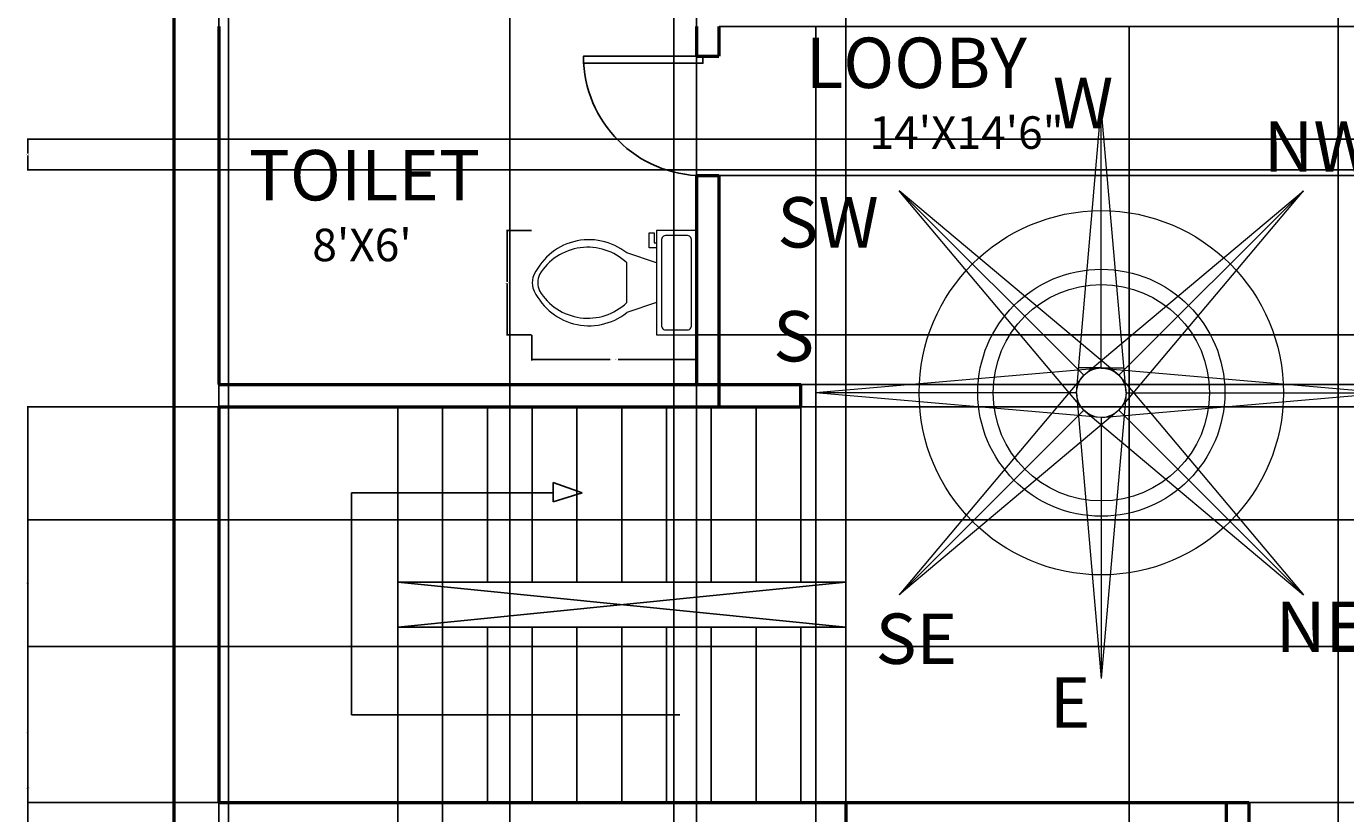
# Model space of a CAD drawing. Units: inches. Extents: x 19425 to 19848, y 45806 to 46417.
# Tile 3 of 5: x 19425 to 19690, y 45967 to 46125. Entities that reach past the tile are written whole.
import ezdxf

# ---------------------------------------------------------------- set-up
doc = ezdxf.new("R2010")
doc.units = ezdxf.units.IN
for name, color, linetype, lineweight in [('A-ANNO-DIMS', 2, 'Continuous', 18), ('A-ANNO-SYMB', 3, 'Continuous', 18), ('A-AREA-IDEN', 3, 'Continuous', 25), ('A-FLOR-FIXT', 2, 'Continuous', 20), ('door', 4, 'Continuous', 25), ('furniture', 2, 'Continuous', 18), ('staircase', 7, 'Continuous', 25), ('wall', 6, 'Continuous', 50)]:
    doc.layers.add(name, color=color, linetype=linetype, lineweight=lineweight)
doc.styles.get("Standard").update_dxf_attribs({"font": 'arial.ttf'})
doc.dimstyles.get("Standard").update_dxf_attribs({"dimtxt": 0.18, "dimasz": 0.18, "dimexe": 0.18, "dimexo": 0.0625, "dimgap": 0.09, "dimtad": 0, "dimtih": 1, "dimtoh": 1, "dimdec": 4, "dimzin": 0, "dimdsep": 46, "dimtxsty": 'Standard', "dimcen": 0.09, "dimadec": 0, "dimazin": 0, "dimtfac": 1, "dimtdec": 4, "dimtofl": 0, "dimtmove": 0, "dimatfit": 3, "dimfxl": 1, "dimtolj": 1, "dimtzin": 0, "dimarcsym": 0})

# ---------------------------------------------------------------- blocks, each defined once
blk = doc.blocks.new('*U2')
for p, q in [((0, 0), (0, -100)), ((750, 0), (750, -100))]:
    blk.add_line(p, q)
blk.add_lwpolyline([(0, 0), (0, 750), (43.75, 750), (43.75, 0)], close=True)
blk.add_arc((0, 0), 750, 0, 90)
blk = doc.blocks.new('Toilet - top')
for p, q in [((9.5, -6), (9.5, -2)), ((-10, -8.5), (-8, -8.5)), ((-10, -9.5), (-10, -8.5)), ((-7, -9.5), (-10, -9.5)), ((-8, -8.5), (-8, -8)), ((-7, -8), (-7, -9.5)), ((-4, -8), (-6, -14)), ((4, -8), (6, -14)), ((4, -14), (-4, -14))]:
    blk.add_line(p, q)
blk.add_lwpolyline([(10.5, -8), (10.5, 0), (-10.5, 0), (-10.5, -8)], close=True)
for points in [[(-9.5, -2), (-9.5, -6)], [(8.5, -1), (-8.5, -1)], [(-8.5, -7), (8.5, -7)]]:
    blk.add_lwpolyline(points)
for centre, radius, start, end in [((-8.62, -1.88), 0.884, 81.8699, 188.1301), ((8.62, -1.88), 0.884, 351.8699, 98.1301), ((-8.62, -6.12), 0.884, 171.8699, 278.1301), ((8.62, -6.12), 0.884, 261.8699, 8.1301), ((3.52, -21.58), 12.17, 141.4691, 247.9714), ((4.2, -21.82), 11.33, 136.3677, 238.9468), ((-3.52, -21.58), 12.17, 292.0284, 38.5307), ((-4.2, -21.82), 11.33, 301.053, 43.6321), ((0, -27.88), 4, 245.7318, 294.2682), ((0, -29), 4, 254.8605, 285.1395)]:
    blk.add_arc(centre, radius, start, end)
blk = doc.blocks.new('*U7')
at = {"layer": 'furniture'}
for p in [(-4.98, -28.71), (0, -23.73), (4.98, -28.71)]:
    blk.add_line(p, (0, 28.71), dxfattribs=at)
blk = doc.blocks.new('*U8')
at = {"layer": 'A-ANNO-SYMB', "transparency": 16777216}
blk.add_blockref('*U7', (19641.16, 46080.31), dxfattribs=at)
for p, rotation in [((19620.86, 46071.91), 45.00000000000001), ((19661.46, 46071.91), 315), ((19612.45, 46051.6), 90), ((19669.87, 46051.6), 270.0000000000001), ((19620.86, 46031.3), 135), ((19661.46, 46031.3), 225), ((19641.16, 46022.9), 180)]:
    blk.add_blockref('*U7', p, dxfattribs=dict(at, rotation=rotation))
blk = doc.blocks.new('*D18')
at = {"layer": 'A-ANNO-DIMS', "color": 0, "lineweight": -2, "transparency": 16777216}
for p, q in [((19526.73, 46063.16), (19526.73, 46058.08)), ((19559.78, 46063.16), (19559.78, 46058.08)), ((19526.91, 46058.26), (19542.48, 46058.26)), ((19559.6, 46058.26), (19544.03, 46058.26))]:
    blk.add_line(p, q, dxfattribs=at)
at = {"layer": 'A-ANNO-DIMS', "color": 0, "transparency": 16777216}
for points in [[(19526.91, 46058.29), (19526.91, 46058.23), (19526.73, 46058.26)], [(19559.6, 46058.29), (19559.6, 46058.23), (19559.78, 46058.26)]]:
    blk.add_solid(points, dxfattribs=at)
at = {"layer": 'Defpoints', "color": 0, "transparency": 16777216}
for p in [(19526.73, 46063.22), (19559.78, 46063.22), (19559.78, 46058.26)]:
    blk.add_point(p, dxfattribs=at)
at = {"layer": 'A-ANNO-DIMS', "color": 0, "transparency": 16777216, "insert": (19543.26, 46058.26), "char_height": 0.18, "attachment_point": 5}
blk.add_mtext('\\A1;WC 33 TYP.', dxfattribs=at)
blk = doc.blocks.new('*D19')
at = {"layer": 'A-ANNO-DIMS', "color": 0, "lineweight": -2, "transparency": 16777216}
for p, q in [((19526.67, 46084.22), (19521.6, 46084.22)), ((19521.78, 46084.04), (19521.78, 46073.9)), ((19521.78, 46063.4), (19521.78, 46073.54)), ((19526.67, 46063.22), (19521.6, 46063.22))]:
    blk.add_line(p, q, dxfattribs=at)
at = {"layer": 'A-ANNO-DIMS', "color": 0, "transparency": 16777216}
for points in [[(19521.75, 46084.04), (19521.81, 46084.04), (19521.78, 46084.22)], [(19521.75, 46063.4), (19521.81, 46063.4), (19521.78, 46063.22)]]:
    blk.add_solid(points, dxfattribs=at)
at = {"layer": 'Defpoints', "color": 0, "transparency": 16777216}
for p in [(19526.73, 46084.22), (19521.78, 46063.22), (19526.73, 46063.22)]:
    blk.add_point(p, dxfattribs=at)
at = {"layer": 'A-ANNO-DIMS', "color": 0, "transparency": 16777216, "insert": (19521.78, 46073.72), "char_height": 0.18, "attachment_point": 5}
blk.add_mtext('\\A1;21 TYP.', dxfattribs=at)
blk = doc.blocks.new('*D34')
at = {"layer": 'A-ANNO-DIMS', "color": 0, "lineweight": -2, "transparency": 16777216}
for p, q in [((19463.78, 46303.69), (19463.78, 45806.22)), ((19522.3, 46304.14), (19522.3, 45806.22)), ((19463.96, 45806.4), (19492.65, 45806.4)), ((19522.12, 45806.4), (19493.43, 45806.4))]:
    blk.add_line(p, q, dxfattribs=at)
at = {"layer": 'A-ANNO-DIMS', "color": 0, "transparency": 16777216}
for points in [[(19463.96, 45806.43), (19463.96, 45806.37), (19463.78, 45806.4)], [(19522.12, 45806.43), (19522.12, 45806.37), (19522.3, 45806.4)]]:
    blk.add_solid(points, dxfattribs=at)
at = {"layer": 'Defpoints', "color": 0, "transparency": 16777216}
for p in [(19463.78, 46303.75), (19522.3, 46304.2), (19522.3, 45806.4)]:
    blk.add_point(p, dxfattribs=at)
at = {"layer": 'A-ANNO-DIMS', "color": 0, "transparency": 16777216, "insert": (19493.04, 45806.4), "char_height": 0.18, "attachment_point": 5}
blk.add_mtext('\\A1;58.52', dxfattribs=at)
blk = doc.blocks.new('*D44')
at = {"layer": 'A-ANNO-DIMS', "color": 0, "lineweight": -2, "transparency": 16777216}
for p, q in [((19463.78, 45969.32), (19463.78, 46342.28)), ((19589.78, 45969.32), (19589.78, 46342.28)), ((19463.96, 46342.1), (19526.5, 46342.1)), ((19589.6, 46342.1), (19527.06, 46342.1))]:
    blk.add_line(p, q, dxfattribs=at)
at = {"layer": 'A-ANNO-DIMS', "color": 0, "transparency": 16777216}
for points in [[(19463.96, 46342.13), (19463.96, 46342.07), (19463.78, 46342.1)], [(19589.6, 46342.13), (19589.6, 46342.07), (19589.78, 46342.1)]]:
    blk.add_solid(points, dxfattribs=at)
at = {"layer": 'Defpoints', "color": 0, "transparency": 16777216}
for p in [(19589.78, 46342.1), (19463.78, 45969.25), (19589.78, 45969.25)]:
    blk.add_point(p, dxfattribs=at)
at = {"layer": 'A-ANNO-DIMS', "color": 0, "transparency": 16777216, "insert": (19526.78, 46342.1), "char_height": 0.18, "attachment_point": 5}
blk.add_mtext('\\A1;126', dxfattribs=at)
blk = doc.blocks.new('*D45')
at = {"layer": 'A-ANNO-DIMS', "color": 0, "lineweight": -2, "transparency": 16777216}
for p, q in [((19463.72, 46048.75), (19425.25, 46048.75)), ((19425.43, 46048.57), (19425.43, 46009.19)), ((19425.43, 45969.43), (19425.43, 46008.82)), ((19463.72, 45969.25), (19425.25, 45969.25))]:
    blk.add_line(p, q, dxfattribs=at)
at = {"layer": 'A-ANNO-DIMS', "color": 0, "transparency": 16777216}
for points in [[(19425.4, 46048.57), (19425.46, 46048.57), (19425.43, 46048.75)], [(19425.4, 45969.43), (19425.46, 45969.43), (19425.43, 45969.25)]]:
    blk.add_solid(points, dxfattribs=at)
at = {"layer": 'Defpoints', "color": 0, "transparency": 16777216}
for p in [(19425.43, 46048.75), (19463.78, 46048.75), (19463.78, 45969.25)]:
    blk.add_point(p, dxfattribs=at)
at = {"layer": 'A-ANNO-DIMS', "color": 0, "transparency": 16777216, "insert": (19425.43, 46009), "char_height": 0.18, "attachment_point": 5}
blk.add_mtext('\\A1;79.5', dxfattribs=at)
blk = doc.blocks.new('*D46')
at = {"layer": 'A-ANNO-DIMS', "color": 0, "lineweight": -2, "transparency": 16777216}
for p, q in [((19646.78, 46125.19), (19646.78, 45806.22)), ((19688.78, 46125.19), (19688.78, 45806.22)), ((19646.96, 45806.4), (19667.56, 45806.4)), ((19688.6, 45806.4), (19668, 45806.4))]:
    blk.add_line(p, q, dxfattribs=at)
at = {"layer": 'A-ANNO-DIMS', "color": 0, "transparency": 16777216}
for points in [[(19646.96, 45806.43), (19646.96, 45806.37), (19646.78, 45806.4)], [(19688.6, 45806.43), (19688.6, 45806.37), (19688.78, 45806.4)]]:
    blk.add_solid(points, dxfattribs=at)
at = {"layer": 'Defpoints', "color": 0, "transparency": 16777216}
for p in [(19646.78, 46125.25), (19688.78, 46125.25), (19688.78, 45806.4)]:
    blk.add_point(p, dxfattribs=at)
at = {"layer": 'A-ANNO-DIMS', "color": 0, "transparency": 16777216, "insert": (19667.78, 45806.4), "char_height": 0.18, "attachment_point": 5}
blk.add_mtext('\\A1;42', dxfattribs=at)
blk = doc.blocks.new('*D52')
at = {"layer": 'A-ANNO-DIMS', "color": 0, "lineweight": -2, "transparency": 16777216}
for p, q in [((19732.81, 46000.63), (19425.25, 46000.63)), ((19425.43, 46000.45), (19425.43, 45972.3)), ((19425.43, 45943.79), (19425.43, 45971.94)), ((19732.81, 45943.61), (19425.25, 45943.61))]:
    blk.add_line(p, q, dxfattribs=at)
at = {"layer": 'A-ANNO-DIMS', "color": 0, "transparency": 16777216}
for points in [[(19425.4, 46000.45), (19425.46, 46000.45), (19425.43, 46000.63)], [(19425.4, 45943.79), (19425.46, 45943.79), (19425.43, 45943.61)]]:
    blk.add_solid(points, dxfattribs=at)
at = {"layer": 'Defpoints', "color": 0, "transparency": 16777216}
for p in [(19425.43, 46000.63), (19732.87, 46000.63), (19732.87, 45943.61)]:
    blk.add_point(p, dxfattribs=at)
at = {"layer": 'A-ANNO-DIMS', "color": 0, "transparency": 16777216, "insert": (19425.43, 45972.12), "char_height": 0.18, "attachment_point": 5}
blk.add_mtext('\\A1;57.02', dxfattribs=at)
blk = doc.blocks.new('*D54')
at = {"layer": 'A-ANNO-DIMS', "color": 0, "lineweight": -2, "transparency": 16777216}
for p, q in [((19808.72, 46048.75), (19425.25, 46048.75)), ((19425.43, 46048.57), (19425.43, 45983.58)), ((19425.43, 45918.22), (19425.43, 45983.22)), ((19808.72, 45918.04), (19425.25, 45918.04))]:
    blk.add_line(p, q, dxfattribs=at)
at = {"layer": 'A-ANNO-DIMS', "color": 0, "transparency": 16777216}
for points in [[(19425.4, 46048.57), (19425.46, 46048.57), (19425.43, 46048.75)], [(19425.4, 45918.22), (19425.46, 45918.22), (19425.43, 45918.04)]]:
    blk.add_solid(points, dxfattribs=at)
at = {"layer": 'Defpoints', "color": 0, "transparency": 16777216}
for p in [(19425.43, 46048.75), (19808.78, 46048.75), (19808.78, 45918.04)]:
    blk.add_point(p, dxfattribs=at)
at = {"layer": 'A-ANNO-DIMS', "color": 0, "transparency": 16777216, "insert": (19425.43, 45983.4), "char_height": 0.18, "attachment_point": 5}
blk.add_mtext('\\A1;130.7', dxfattribs=at)
blk = doc.blocks.new('*D59')
at = {"layer": 'A-ANNO-DIMS', "color": 0, "lineweight": -2, "transparency": 16777216}
for p, q in [((19463.78, 45868.98), (19463.78, 46342.28)), ((19465.72, 45866.97), (19465.72, 46342.28)), ((19463.96, 46342.1), (19464.36, 46342.1)), ((19465.54, 46342.1), (19465.14, 46342.1))]:
    blk.add_line(p, q, dxfattribs=at)
at = {"layer": 'A-ANNO-DIMS', "color": 0, "transparency": 16777216}
for points in [[(19463.96, 46342.13), (19463.96, 46342.07), (19463.78, 46342.1)], [(19465.54, 46342.13), (19465.54, 46342.07), (19465.72, 46342.1)]]:
    blk.add_solid(points, dxfattribs=at)
at = {"layer": 'Defpoints', "color": 0, "transparency": 16777216}
for p in [(19465.72, 46342.1), (19463.78, 45868.92), (19465.72, 45866.91)]:
    blk.add_point(p, dxfattribs=at)
at = {"layer": 'A-ANNO-DIMS', "color": 0, "transparency": 16777216, "insert": (19464.75, 46342.1), "char_height": 0.18, "attachment_point": 5}
blk.add_mtext('\\A1;1.938', dxfattribs=at)
blk = doc.blocks.new('*D60')
at = {"layer": 'A-ANNO-DIMS', "color": 0, "lineweight": -2, "transparency": 16777216}
for p, q in [((19555.24, 45865.14), (19555.24, 46342.28)), ((19559.78, 45868.98), (19559.78, 46342.28)), ((19555.42, 46342.1), (19557.18, 46342.1)), ((19559.6, 46342.1), (19557.84, 46342.1))]:
    blk.add_line(p, q, dxfattribs=at)
at = {"layer": 'A-ANNO-DIMS', "color": 0, "transparency": 16777216}
for points in [[(19555.42, 46342.13), (19555.42, 46342.07), (19555.24, 46342.1)], [(19559.6, 46342.13), (19559.6, 46342.07), (19559.78, 46342.1)]]:
    blk.add_solid(points, dxfattribs=at)
at = {"layer": 'Defpoints', "color": 0, "transparency": 16777216}
for p in [(19559.78, 46342.1), (19559.78, 45868.92), (19555.24, 45865.08)]:
    blk.add_point(p, dxfattribs=at)
at = {"layer": 'A-ANNO-DIMS', "color": 0, "transparency": 16777216, "insert": (19557.51, 46342.1), "char_height": 0.18, "attachment_point": 5}
blk.add_mtext('\\A1;4.54', dxfattribs=at)
blk = doc.blocks.new('*D63')
at = {"layer": 'A-ANNO-DIMS', "color": 0, "lineweight": -2, "transparency": 16777216}
for p, q in [((19463.78, 46125.19), (19463.78, 45806.22)), ((19583.78, 46125.19), (19583.78, 45806.22)), ((19463.96, 45806.4), (19523.5, 45806.4)), ((19583.6, 45806.4), (19524.06, 45806.4))]:
    blk.add_line(p, q, dxfattribs=at)
at = {"layer": 'A-ANNO-DIMS', "color": 0, "transparency": 16777216}
for points in [[(19463.96, 45806.43), (19463.96, 45806.37), (19463.78, 45806.4)], [(19583.6, 45806.43), (19583.6, 45806.37), (19583.78, 45806.4)]]:
    blk.add_solid(points, dxfattribs=at)
at = {"layer": 'Defpoints', "color": 0, "transparency": 16777216}
for p in [(19463.78, 46125.25), (19583.78, 46125.25), (19583.78, 45806.4)]:
    blk.add_point(p, dxfattribs=at)
at = {"layer": 'A-ANNO-DIMS', "color": 0, "transparency": 16777216, "insert": (19523.78, 45806.4), "char_height": 0.18, "attachment_point": 5}
blk.add_mtext('\\A1;120', dxfattribs=at)
blk = doc.blocks.new('*D64')
at = {"layer": 'A-ANNO-DIMS', "color": 0, "lineweight": -2, "transparency": 16777216}
for p, q in [((19463.78, 46048.69), (19463.78, 45806.22)), ((19499.78, 46048.69), (19499.78, 45806.22)), ((19463.96, 45806.4), (19481.56, 45806.4)), ((19499.6, 45806.4), (19482, 45806.4))]:
    blk.add_line(p, q, dxfattribs=at)
at = {"layer": 'A-ANNO-DIMS', "color": 0, "transparency": 16777216}
for points in [[(19463.96, 45806.43), (19463.96, 45806.37), (19463.78, 45806.4)], [(19499.6, 45806.43), (19499.6, 45806.37), (19499.78, 45806.4)]]:
    blk.add_solid(points, dxfattribs=at)
at = {"layer": 'Defpoints', "color": 0, "transparency": 16777216}
for p in [(19463.78, 46048.75), (19499.78, 46048.75), (19499.78, 45806.4)]:
    blk.add_point(p, dxfattribs=at)
at = {"layer": 'A-ANNO-DIMS', "color": 0, "transparency": 16777216, "insert": (19481.78, 45806.4), "char_height": 0.18, "attachment_point": 5}
blk.add_mtext('\\A1;36', dxfattribs=at)
blk = doc.blocks.new('*D65')
at = {"layer": 'A-ANNO-DIMS', "color": 0, "lineweight": -2, "transparency": 16777216}
for p, q in [((19499.78, 46048.69), (19499.78, 45806.22)), ((19508.78, 46048.69), (19508.78, 45806.22)), ((19499.96, 45806.4), (19504.13, 45806.4)), ((19508.6, 45806.4), (19504.43, 45806.4))]:
    blk.add_line(p, q, dxfattribs=at)
at = {"layer": 'A-ANNO-DIMS', "color": 0, "transparency": 16777216}
for points in [[(19499.96, 45806.43), (19499.96, 45806.37), (19499.78, 45806.4)], [(19508.6, 45806.43), (19508.6, 45806.37), (19508.78, 45806.4)]]:
    blk.add_solid(points, dxfattribs=at)
at = {"layer": 'Defpoints', "color": 0, "transparency": 16777216}
for p in [(19499.78, 46048.75), (19508.78, 46048.75), (19508.78, 45806.4)]:
    blk.add_point(p, dxfattribs=at)
at = {"layer": 'A-ANNO-DIMS', "color": 0, "transparency": 16777216, "insert": (19504.28, 45806.4), "char_height": 0.18, "attachment_point": 5}
blk.add_mtext('\\A1;9', dxfattribs=at)
blk = doc.blocks.new('*D66')
at = {"layer": 'A-ANNO-DIMS', "color": 0, "lineweight": -2, "transparency": 16777216}
for p, q in [((19559.84, 46063.22), (19847.31, 46063.22)), ((19847.13, 46063.04), (19847.13, 46058.42)), ((19847.13, 46053.43), (19847.13, 46058.06)), ((19559.84, 46053.25), (19847.31, 46053.25))]:
    blk.add_line(p, q, dxfattribs=at)
at = {"layer": 'A-ANNO-DIMS', "color": 0, "transparency": 16777216}
for points in [[(19847.1, 46063.04), (19847.16, 46063.04), (19847.13, 46063.22)], [(19847.1, 46053.43), (19847.16, 46053.43), (19847.13, 46053.25)]]:
    blk.add_solid(points, dxfattribs=at)
at = {"layer": 'Defpoints', "color": 0, "transparency": 16777216}
for p in [(19559.78, 46063.22), (19847.13, 46063.22), (19559.78, 46053.25)]:
    blk.add_point(p, dxfattribs=at)
at = {"layer": 'A-ANNO-DIMS', "color": 0, "transparency": 16777216, "insert": (19847.13, 46058.24), "char_height": 0.18, "attachment_point": 5}
blk.add_mtext('\\A1;9.967', dxfattribs=at)
blk = doc.blocks.new('*D67')
at = {"layer": 'A-ANNO-DIMS', "color": 0, "lineweight": -2, "transparency": 16777216}
for p, q in [((19564.34, 46125.25), (19847.31, 46125.25)), ((19847.13, 46125.07), (19847.13, 46110.44)), ((19847.13, 46095.43), (19847.13, 46110.07)), ((19564.34, 46095.25), (19847.31, 46095.25))]:
    blk.add_line(p, q, dxfattribs=at)
at = {"layer": 'A-ANNO-DIMS', "color": 0, "transparency": 16777216}
for points in [[(19847.1, 46125.07), (19847.16, 46125.07), (19847.13, 46125.25)], [(19847.1, 46095.43), (19847.16, 46095.43), (19847.13, 46095.25)]]:
    blk.add_solid(points, dxfattribs=at)
at = {"layer": 'Defpoints', "color": 0, "transparency": 16777216}
for p in [(19564.28, 46125.25), (19847.13, 46125.25), (19564.28, 46095.25)]:
    blk.add_point(p, dxfattribs=at)
at = {"layer": 'A-ANNO-DIMS', "color": 0, "transparency": 16777216, "insert": (19847.13, 46110.25), "char_height": 0.18, "attachment_point": 5}
blk.add_mtext('\\A1;30', dxfattribs=at)
blk = doc.blocks.new('*D69')
at = {"layer": 'A-ANNO-DIMS', "color": 0, "lineweight": -2, "transparency": 16777216}
for p, q in [((19787.22, 46026.07), (19425.25, 46026.07)), ((19425.43, 46025.89), (19425.43, 46013.53)), ((19425.43, 46000.81), (19425.43, 46013.17)), ((19768.15, 46000.63), (19425.25, 46000.63))]:
    blk.add_line(p, q, dxfattribs=at)
at = {"layer": 'A-ANNO-DIMS', "color": 0, "transparency": 16777216}
for points in [[(19425.4, 46025.89), (19425.46, 46025.89), (19425.43, 46026.07)], [(19425.4, 46000.81), (19425.46, 46000.81), (19425.43, 46000.63)]]:
    blk.add_solid(points, dxfattribs=at)
at = {"layer": 'Defpoints', "color": 0, "transparency": 16777216}
for p in [(19425.43, 46026.07), (19787.29, 46026.07), (19768.22, 46000.63)]:
    blk.add_point(p, dxfattribs=at)
at = {"layer": 'A-ANNO-DIMS', "color": 0, "transparency": 16777216, "insert": (19425.43, 46013.35), "char_height": 0.18, "attachment_point": 5}
blk.add_mtext('\\A1;25.44', dxfattribs=at)
blk = doc.blocks.new('*D70')
at = {"layer": 'A-ANNO-DIMS', "color": 0, "lineweight": -2, "transparency": 16777216}
for p, q in [((19666.34, 45969.25), (19847.31, 45969.25)), ((19847.13, 45969.07), (19847.13, 45907.19)), ((19847.13, 45844.93), (19847.13, 45906.82)), ((19666.34, 45844.75), (19847.31, 45844.75))]:
    blk.add_line(p, q, dxfattribs=at)
at = {"layer": 'A-ANNO-DIMS', "color": 0, "transparency": 16777216}
for points in [[(19847.1, 45969.07), (19847.16, 45969.07), (19847.13, 45969.25)], [(19847.1, 45844.93), (19847.16, 45844.93), (19847.13, 45844.75)]]:
    blk.add_solid(points, dxfattribs=at)
at = {"layer": 'Defpoints', "color": 0, "transparency": 16777216}
for p in [(19666.28, 45969.25), (19847.13, 45969.25), (19666.28, 45844.75)]:
    blk.add_point(p, dxfattribs=at)
at = {"layer": 'A-ANNO-DIMS', "color": 0, "transparency": 16777216, "insert": (19847.13, 45907), "char_height": 0.18, "attachment_point": 5}
blk.add_mtext('\\A1;124.5', dxfattribs=at)
blk = doc.blocks.new('*D74')
at = {"layer": 'A-ANNO-DIMS', "color": 0, "lineweight": -2, "transparency": 16777216}
for p, q in [((19688.78, 46129.69), (19688.78, 45806.22)), ((19778.78, 46129.69), (19778.78, 45806.22)), ((19688.96, 45806.4), (19733.56, 45806.4)), ((19778.6, 45806.4), (19734, 45806.4))]:
    blk.add_line(p, q, dxfattribs=at)
at = {"layer": 'A-ANNO-DIMS', "color": 0, "transparency": 16777216}
for points in [[(19688.96, 45806.43), (19688.96, 45806.37), (19688.78, 45806.4)], [(19778.6, 45806.43), (19778.6, 45806.37), (19778.78, 45806.4)]]:
    blk.add_solid(points, dxfattribs=at)
at = {"layer": 'Defpoints', "color": 0, "transparency": 16777216}
for p in [(19688.78, 46129.75), (19778.78, 46129.75), (19778.78, 45806.4)]:
    blk.add_point(p, dxfattribs=at)
at = {"layer": 'A-ANNO-DIMS', "color": 0, "transparency": 16777216, "insert": (19733.78, 45806.4), "char_height": 0.18, "attachment_point": 5}
blk.add_mtext('\\A1;90', dxfattribs=at)
blk = doc.blocks.new('*D75')
at = {"layer": 'A-ANNO-DIMS', "color": 0, "lineweight": -2, "transparency": 16777216}
for p, q in [((19802.72, 46102.55), (19425.25, 46102.55)), ((19425.43, 46102.37), (19425.43, 46099.67)), ((19425.43, 46096.6), (19425.43, 46099.31)), ((19800.72, 46096.42), (19425.25, 46096.42))]:
    blk.add_line(p, q, dxfattribs=at)
at = {"layer": 'A-ANNO-DIMS', "color": 0, "transparency": 16777216}
for points in [[(19425.4, 46102.37), (19425.46, 46102.37), (19425.43, 46102.55)], [(19425.4, 46096.6), (19425.46, 46096.6), (19425.43, 46096.42)]]:
    blk.add_solid(points, dxfattribs=at)
at = {"layer": 'Defpoints', "color": 0, "transparency": 16777216}
for p in [(19802.78, 46102.55), (19425.43, 46096.42), (19800.78, 46096.42)]:
    blk.add_point(p, dxfattribs=at)
at = {"layer": 'A-ANNO-DIMS', "color": 0, "transparency": 16777216, "insert": (19425.43, 46099.49), "char_height": 0.18, "attachment_point": 5}
blk.add_mtext('\\A1;6.134', dxfattribs=at)

msp = doc.modelspace()

# ---------------------------------------------------------------- linework, layer by layer
at = {"layer": 'A-ANNO-SYMB'}
for q in [(19636.6092, 46056.5875), (19645.7096, 46056.5875)]:
    msp.add_line((19641.1594, 46056.5875), q, dxfattribs=at)
for radius in [36.614, 36.614, 36.614, 24.8225, 21.7425, 4.9825]:
    msp.add_circle((19641.1594, 46051.6049), radius, dxfattribs=at)
at = {"layer": 'staircase'}
for p, q in [((19499.7812, 46048.7547), (19499.7812, 46013.5047)), ((19508.7812, 46048.7547), (19508.7812, 46013.5047)), ((19517.7812, 46048.7547), (19517.7812, 46013.5047)), ((19526.7812, 46048.7547), (19526.7812, 46013.5047)), ((19535.7812, 46048.7547), (19535.7812, 46013.5047)), ((19544.7812, 46048.7547), (19544.7812, 46013.5047)), ((19553.7812, 46048.7547), (19553.7812, 46013.5047)), ((19562.7812, 46048.7547), (19562.7812, 46013.5047)), ((19571.7812, 46048.7547), (19571.7812, 46013.5047)), ((19580.7812, 46048.7547), (19580.7812, 46013.5047)), ((19530.9825, 46031.4751), (19530.9825, 46033.5787)), ((19530.9825, 46033.5787), (19530.9825, 46029.6728)), ((19530.9825, 46033.5787), (19536.8487, 46031.4751)), ((19490.4933, 45986.8402), (19490.4933, 46031.4751)), ((19490.4933, 46031.4751), (19530.9825, 46031.4751)), ((19530.9825, 46029.6728), (19536.8487, 46031.4751)), ((19589.7812, 46013.5047), (19499.7812, 46013.5047)), ((19499.7812, 46013.5047), (19499.7812, 45969.2547)), ((19499.7812, 46013.5047), (19589.7812, 46004.5047)), ((19499.7812, 46004.5047), (19589.7812, 46013.5047)), ((19589.7812, 46013.5047), (19589.7812, 46004.5047)), ((19589.7812, 46004.5047), (19499.7812, 46004.5047)), ((19508.7812, 46004.5047), (19508.7812, 45969.2547)), ((19517.7812, 46004.5047), (19517.7812, 45969.2547)), ((19526.7812, 46004.5047), (19526.7812, 45969.2547)), ((19535.7812, 46004.5047), (19535.7812, 45969.2547)), ((19544.7812, 46004.5047), (19544.7812, 45969.2547)), ((19553.7812, 46004.5047), (19553.7812, 45969.2547)), ((19562.7812, 46004.5047), (19562.7812, 45969.2547)), ((19571.7812, 46004.5047), (19571.7812, 45969.2547)), ((19580.7812, 46004.5047), (19580.7812, 45969.2547)), ((19589.7812, 46004.5047), (19589.7812, 45969.2547)), ((19556.4435, 45986.8402), (19490.4933, 45986.8402))]:
    msp.add_line(p, q, dxfattribs=at)
at = {"layer": 'wall'}
for p, q in [((19454.7812, 46312.7547), (19454.7812, 45835.7547)), ((19463.7812, 46125.2547), (19463.7812, 46053.2547)), ((19559.7812, 46125.2547), (19559.7812, 46119.2547)), ((19564.2812, 46125.2547), (19564.2812, 46119.2547)), ((19559.7812, 46119.2547), (19564.2812, 46119.2547)), ((19559.7812, 46095.2547), (19564.2812, 46095.2547)), ((19559.7812, 46095.2547), (19559.7812, 46053.2547)), ((19564.2812, 46095.2547), (19564.2812, 46048.7547)), ((19463.7812, 46053.2547), (19580.7812, 46053.2547)), ((19580.7812, 46048.7547), (19580.7812, 46053.2547)), ((19463.7812, 46048.7547), (19580.7812, 46048.7547)), ((19463.7812, 46048.7547), (19463.7812, 45969.2547)), ((19463.7812, 45969.2547), (19670.7812, 45969.2547)), ((19589.7812, 45969.2547), (19589.7812, 45964.7547)), ((19666.2812, 45969.2547), (19666.2812, 45844.7547)), ((19670.7812, 45969.2547), (19670.7812, 45844.7547))]:
    msp.add_line(p, q, dxfattribs=at)

# ---------------------------------------------------------------- block references
at = {"layer": 'A-ANNO-SYMB'}
msp.add_blockref('*U8', (0, 0), dxfattribs=at)
at = {"layer": 'A-FLOR-FIXT', "rotation": 270}
msp.add_blockref('Toilet - top', (19559.7812, 46073.7218), dxfattribs=at)
at = {"layer": 'door', "xscale": -0.0320000000000009, "yscale": 0.0320000000000009, "zscale": 0.0320000000000009, "rotation": 90}
msp.add_blockref('*U2', (19561.0812, 46119.2547), dxfattribs=at)

# ---------------------------------------------------------------- texts
at = {"layer": 'A-ANNO-SYMB'}
for s, height, p in [('W', 10.1286, (19631.4281, 46104.7919)), ('NW', 10.12861, (19673.7783, 46096.0476)), ('SW', 10.12861, (19576.0471, 46080.7958)), ('S', 10.1286, (19575.2234, 46057.905)), ('NE', 10.12861, (19676.2165, 45999.5028)), ('SE', 10.12861, (19595.7876, 45997.1015)), ('E', 10.1286, (19630.812, 45984.2512))]:
    msp.add_text(s, height=height, dxfattribs=at).set_placement(p)
at = {"layer": 'A-AREA-IDEN'}
for s, height, p in [('LOOBY', 10.12861, (19581.7796, 46112.865)), ('14\'X14\'6"', 6.53608, (19594.5599, 46100.6389)), ('TOILET', 10.12861, (19469.8117, 46090.274)), ("8'X6'", 6.53608, (19482.592, 46078.048))]:
    msp.add_text(s, height=height, dxfattribs=at).set_placement(p)

# ---------------------------------------------------------------- dimensions: what is measured, and where the dimension line sits
at = {"layer": 'A-ANNO-DIMS'}
for base, p1, p2, override, picture, middle in [((19589.7812, 46342.1047), (19463.7812, 45969.2547), (19589.7812, 45969.2547), {"dimdec": 0, "dimlfac": 1, "dimrnd": 0, "dimzin": 0, "dimdsep": 46, "dimlunit": 2}, '*D44', (19526.7812, 46342.1047)), ((19465.7192, 46342.1047), (19463.7812, 45868.9163), (19465.7192, 45866.9088), {"dimdec": 3, "dimlfac": 1, "dimrnd": 0, "dimzin": 0, "dimdsep": 46, "dimlunit": 2}, '*D59', (19464.7502, 46342.1047)), ((19559.7812, 46342.1047), (19555.2409, 45865.0758), (19559.7812, 45868.9163), {"dimdec": 2, "dimlfac": 1, "dimrnd": 0, "dimzin": 0, "dimdsep": 46, "dimlunit": 2}, '*D60', (19557.511, 46342.1047)), ((19522.3015, 45806.4047), (19463.7812, 46303.7547), (19522.3015, 46304.1988), {"dimdec": 2, "dimlfac": 1, "dimrnd": 0, "dimzin": 0, "dimdsep": 46, "dimlunit": 2}, '*D34', (19493.0413, 45806.4047)), ((19778.7812, 45806.4047), (19688.7812, 46129.7547), (19778.7812, 46129.7547), {"dimdec": 0, "dimlfac": 1, "dimrnd": 0, "dimzin": 0, "dimdsep": 46, "dimlunit": 2}, '*D74', (19733.7812, 45806.4047)), ((19583.7812, 45806.4047), (19463.7812, 46125.2547), (19583.7812, 46125.2547), {"dimdec": 0, "dimlfac": 1, "dimrnd": 0, "dimzin": 0, "dimdsep": 46, "dimlunit": 2}, '*D63', (19523.7812, 45806.4047)), ((19688.7812, 45806.4047), (19646.7812, 46125.2547), (19688.7812, 46125.2547), {"dimdec": 0, "dimlfac": 1, "dimrnd": 0, "dimzin": 0, "dimdsep": 46, "dimlunit": 2}, '*D46', (19667.7812, 45806.4047)), ((19499.7812, 45806.4047), (19463.7812, 46048.7547), (19499.7812, 46048.7547), {"dimdec": 0, "dimlfac": 1, "dimrnd": 0, "dimzin": 0, "dimdsep": 46, "dimlunit": 2}, '*D64', (19481.7812, 45806.4047)), ((19508.7812, 45806.4047), (19499.7812, 46048.7547), (19508.7812, 46048.7547), {"dimdec": 0, "dimlfac": 1, "dimrnd": 0, "dimzin": 0, "dimdsep": 46, "dimlunit": 2}, '*D65', (19504.2812, 45806.4047))]:
    dim = msp.add_linear_dim(base=base, p1=p1, p2=p2, dimstyle='Standard', override=override, dxfattribs=at)
    dim.commit()
    dim.dimension.update_dxf_attribs({"geometry": picture, "text_midpoint": middle})
for base, p1, p2, override, picture, middle in [((19847.1312, 46125.2547), (19564.2812, 46095.2547), (19564.2812, 46125.2547), {"dimdec": 0, "dimlfac": 1, "dimrnd": 0, "dimzin": 0, "dimdsep": 46, "dimlunit": 2}, '*D67', (19847.1312, 46110.2547)), ((19425.4312, 46096.4211), (19802.7812, 46102.5547), (19800.7812, 46096.4211), {"dimdec": 3, "dimlfac": 1, "dimrnd": 0, "dimzin": 0, "dimdsep": 46, "dimlunit": 2}, '*D75', (19425.4312, 46099.4879)), ((19847.1312, 46063.2218), (19559.7812, 46053.2547), (19559.7812, 46063.2218), {"dimdec": 3, "dimlfac": 1, "dimrnd": 0, "dimzin": 0, "dimdsep": 46, "dimlunit": 2}, '*D66', (19847.1312, 46058.2382)), ((19425.4312, 46048.7547), (19808.7812, 45918.0438), (19808.7812, 46048.7547), {"dimdec": 1, "dimlfac": 1, "dimrnd": 0, "dimzin": 0, "dimdsep": 46, "dimlunit": 2}, '*D54', (19425.4312, 45983.3992)), ((19425.4312, 46048.7547), (19463.7812, 45969.2547), (19463.7812, 46048.7547), {"dimdec": 1, "dimlfac": 1, "dimrnd": 0, "dimzin": 0, "dimdsep": 46, "dimlunit": 2}, '*D45', (19425.4312, 46009.0047)), ((19425.4312, 46026.0705), (19768.2171, 46000.631), (19787.2853, 46026.0705), {"dimdec": 2, "dimlfac": 1, "dimrnd": 0, "dimzin": 0, "dimdsep": 46, "dimlunit": 2}, '*D69', (19425.4312, 46013.3508)), ((19425.4312, 46000.631), (19732.8741, 45943.6092), (19732.8741, 46000.631), {"dimdec": 2, "dimlfac": 1, "dimrnd": 0, "dimzin": 0, "dimdsep": 46, "dimlunit": 2}, '*D52', (19425.4312, 45972.1201)), ((19847.1312, 45969.2547), (19666.2812, 45844.7547), (19666.2812, 45969.2547), {"dimdec": 1, "dimlfac": 1, "dimrnd": 0, "dimzin": 0, "dimdsep": 46, "dimlunit": 2}, '*D70', (19847.1312, 45907.0047))]:
    dim = msp.add_linear_dim(base=base, p1=p1, p2=p2, angle=90, dimstyle='Standard', override=override, dxfattribs=at)
    dim.commit()
    dim.dimension.update_dxf_attribs({"geometry": picture, "text_midpoint": middle})
dim = msp.add_linear_dim(base=(19521.778, 46063.2218), p1=(19526.7349, 46084.2218), p2=(19526.7349, 46063.2218), angle=270, text='<> TYP.', dimstyle='Standard', override={"dimdec": 0, "dimlfac": 1, "dimrnd": 0, "dimzin": 0, "dimdsep": 46, "dimlunit": 2}, dxfattribs=at)
dim.commit()
dim.dimension.update_dxf_attribs({"geometry": '*D19', "text_midpoint": (19521.778, 46073.7218)})
dim = msp.add_linear_dim(base=(19559.7812, 46058.2648), p1=(19526.7349, 46063.2218), p2=(19559.7812, 46063.2218), text='WC <> TYP.', dimstyle='Standard', override={"dimdec": 0, "dimlfac": 1, "dimrnd": 0, "dimzin": 0, "dimdsep": 46, "dimlunit": 2}, dxfattribs=at)
dim.commit()
dim.dimension.update_dxf_attribs({"geometry": '*D18', "text_midpoint": (19543.258, 46058.2648)})

doc.saveas('drawing.dxf')
